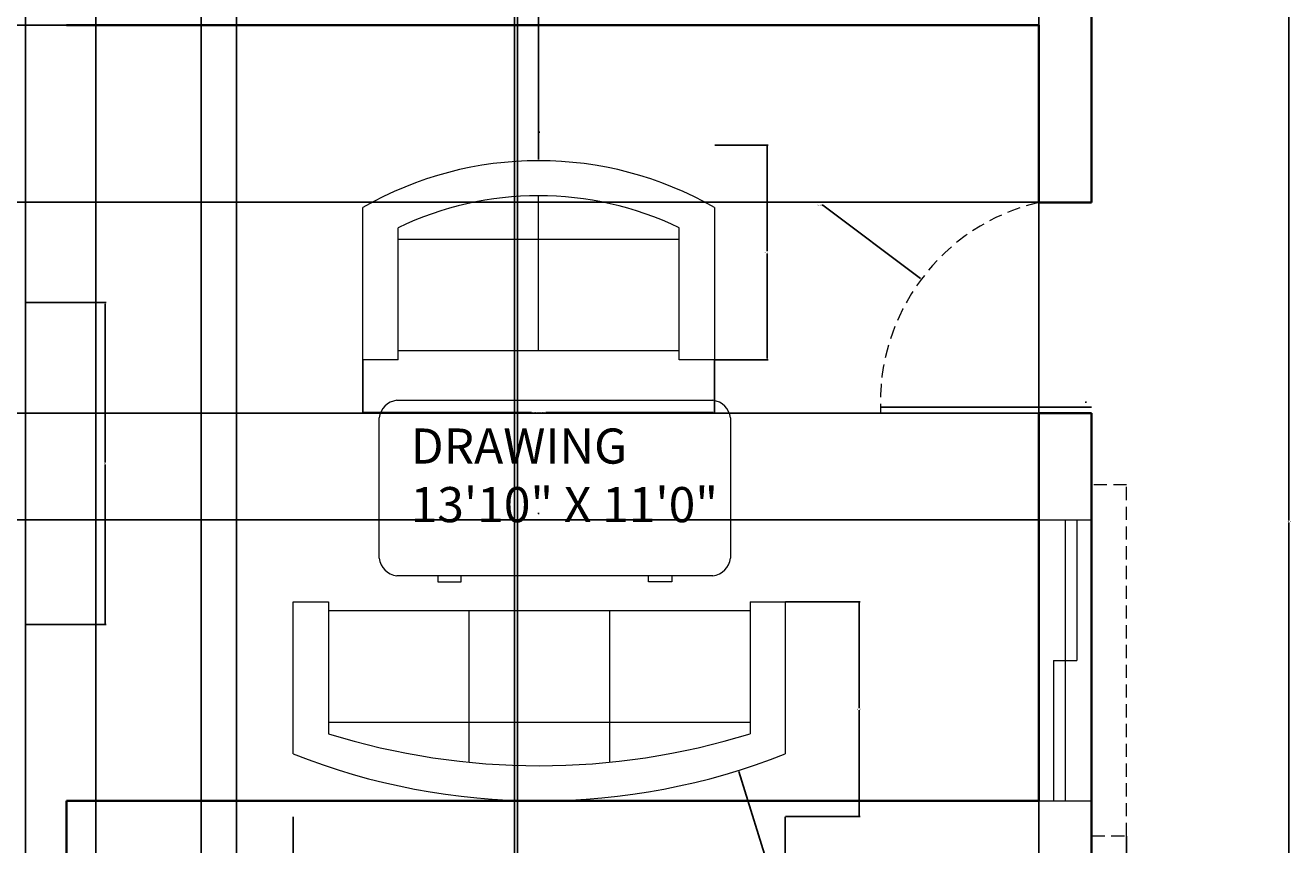
# Model space of a CAD drawing. Units: inches. Extents: x 6662 to 7211, y 5077 to 5683.
# Tile 6 of 9: x 6995 to 7211, y 5325 to 5465. Entities that reach past the tile are written whole.
import ezdxf

# ---------------------------------------------------------------- set-up
doc = ezdxf.new("R2010")
doc.units = ezdxf.units.IN
doc.header["$LTSCALE"] = 3
doc.header["$MEASUREMENT"] = 0
doc.linetypes.add('HIDDEN', pattern=[0.375, 0.25, -0.125])
for name, color, linetype, lineweight in [('A-ANNO-DIMS', 2, 'Continuous', 18), ('A-AREA-IDEN', 7, 'Continuous', 18), ('A-DOOR', 4, 'Continuous', 25), ('A-DOOR-HIDN', 4, 'HIDDEN', 13), ('A-FLOR-CASE-PATT', 241, 'Continuous', 13), ('A-FURN', 8, 'Continuous', 18), ('A-GLAZ', 4, 'Continuous', 18), ('A-GLAZ-OVHD', 4, 'HIDDEN', 13), ('A-WALL', 7, 'Continuous', 35)]:
    doc.layers.add(name, color=color, linetype=linetype, lineweight=lineweight)
doc.styles.get("Standard").update_dxf_attribs({"font": 'arial.ttf'})
doc.dimstyles.get("Standard").update_dxf_attribs({"dimtxt": 0.18, "dimasz": 0.18, "dimexe": 0.18, "dimexo": 0.0625, "dimgap": 0.09, "dimtad": 0, "dimtih": 1, "dimtoh": 1, "dimdec": 4, "dimzin": 0, "dimdsep": 46, "dimtxsty": 'Standard', "dimcen": 0.09, "dimadec": 0, "dimazin": 0, "dimtfac": 1, "dimtdec": 4, "dimtofl": 0, "dimtmove": 0, "dimatfit": 3, "dimfxl": 1, "dimtolj": 1, "dimtzin": 0, "dimarcsym": 0})

# ---------------------------------------------------------------- blocks, each defined once
blk = doc.blocks.new('Sofa - Roundback 7 ft.')
for p, q in [((-12.00002, -32.4421), (-12.00003, -6.5971)), ((11.99997, -32.4421), (11.99998, -6.5971)), ((-36.000027, -34), (-36.000027, -11.4696)), ((35.99998, -34), (35.99998, -11.4696)), ((-35.999844, -13.3819), (35.9998, -13.3819)), ((-36.000027, -32.4421), (35.99998, -32.4421))]:
    blk.add_line(p, q)
for points in [[(-36.000027, -34), (-42.000027, -34), (-42.000027, -8)], [(41.99998, -8), (41.99998, -34), (35.99998, -34)]]:
    blk.add_lwpolyline(points)
for centre, radius, start, end in [((0, -114.25), 114.25, 68.43141, 111.5686), ((-0.00001, -127.1968), 121.1968, 72.72033, 107.2797)]:
    blk.add_arc(centre, radius, start, end)
blk = doc.blocks.new('Desk - 30 x 60 in.')
for p, q in [((-26.999995, 0), (26.999995, 0)), ((-29.999995, -27), (-29.999995, -3)), ((29.999995, -3), (29.999995, -27)), ((26.999995, -30), (-26.999995, -30)), ((-20.000005, -30), (-20.000005, -31)), ((-16.000005, -31), (-16.000005, -30)), ((15.999995, -31), (15.999995, -30)), ((19.999995, -30), (19.999995, -31)), ((-20.000005, -31), (-16.000005, -31)), ((19.999995, -31), (15.999995, -31))]:
    blk.add_line(p, q)
for centre, start, end in [((-26.499995, -3.5), 98.1301, 171.8699), ((26.499995, -3.5), 8.130102, 81.8699), ((-26.499995, -26.5), 188.1301, 261.8699), ((26.499995, -26.5), 278.1301, 351.8699)]:
    blk.add_arc(centre, 3.535534, start, end)
blk = doc.blocks.new('Sofa - Roundback Loveseat 5 ft.')
for p, q in [((0, -32.44198), (0, -5.99998)), ((-24, -33.99998), (-24, -11.46958)), ((24.00004, -33.99998), (24.00004, -11.46958)), ((-23.9998, -13.38178), (23.99986, -13.38178)), ((-24, -32.44198), (24.00004, -32.44198))]:
    blk.add_line(p, q)
for points in [[(-24, -33.99998), (-30, -33.99998), (-30, -7.99998)], [(30.00004, -7.99998), (30.00004, -33.99998), (24.00004, -33.99998)]]:
    blk.add_lwpolyline(points)
for centre, radius, start, end in [((0, -60.24998), 60.24998, 60.13715, 119.8628), ((0, -61.38438), 55.38444, 64.32083, 115.6792)]:
    blk.add_arc(centre, radius, start, end)
blk = doc.blocks.new('WIN-SLIDER-48IN')
for p, q in [((0, 0), (0, 9)), ((48, 0), (48, 9)), ((0, 6.5), (24, 6.5)), ((24, 2.5), (24, 6.5)), ((0, 4.5), (48, 4.5)), ((24, 2.5), (48, 2.5))]:
    blk.add_line(p, q)
blk = doc.blocks.new('WIN-HOOD-48IN')
at = {"ltscale": 3}
for p, q in [((0, 0), (0, 6)), ((0, 6), (54, 6)), ((54, 6), (60, 6)), ((60, 6), (60, 0)), ((6, 0), (0, 0))]:
    blk.add_line(p, q, dxfattribs=at)
blk = doc.blocks.new('*D28')
at = {"layer": 'A-ANNO-DIMS', "color": 0, "lineweight": -2, "ltscale": 3, "transparency": 16777216}
for p, q in [((7040.57, 5329.37), (7040.57, 5316.65)), ((7124.57, 5329.37), (7124.57, 5316.65)), ((7040.75, 5316.83), (7081.66, 5316.83)), ((7124.39, 5316.83), (7083.47, 5316.83))]:
    blk.add_line(p, q, dxfattribs=at)
at = {"layer": 'A-ANNO-DIMS', "color": 0, "ltscale": 3, "transparency": 16777216}
for points in [[(7040.75, 5316.86), (7040.75, 5316.8), (7040.57, 5316.83)], [(7124.39, 5316.86), (7124.39, 5316.8), (7124.57, 5316.83)]]:
    blk.add_solid(points, dxfattribs=at)
at = {"layer": 'Defpoints', "color": 0, "ltscale": 3, "transparency": 16777216}
for p in [(7040.57, 5329.43), (7124.57, 5329.43), (7040.57, 5316.83)]:
    blk.add_point(p, dxfattribs=at)
at = {"layer": 'A-ANNO-DIMS', "color": 0, "ltscale": 3, "transparency": 16777216, "insert": (7082.57, 5316.83), "char_height": 0.18, "attachment_point": 5}
blk.add_mtext('\\A1;SOFA 84 TYP.', dxfattribs=at)
blk = doc.blocks.new('*D29')
at = {"layer": 'A-ANNO-DIMS', "color": 0, "lineweight": -2, "ltscale": 3, "transparency": 16777216}
for p, q in [((7124.63, 5366.1), (7137.35, 5366.1)), ((7137.17, 5365.92), (7137.17, 5347.95)), ((7137.17, 5329.61), (7137.17, 5347.58)), ((7124.63, 5329.43), (7137.35, 5329.43))]:
    blk.add_line(p, q, dxfattribs=at)
at = {"layer": 'A-ANNO-DIMS', "color": 0, "ltscale": 3, "transparency": 16777216}
for points in [[(7137.14, 5365.92), (7137.2, 5365.92), (7137.17, 5366.1)], [(7137.14, 5329.61), (7137.2, 5329.61), (7137.17, 5329.43)]]:
    blk.add_solid(points, dxfattribs=at)
at = {"layer": 'Defpoints', "color": 0, "ltscale": 3, "transparency": 16777216}
for p in [(7124.57, 5366.1), (7124.57, 5329.43), (7137.17, 5329.43)]:
    blk.add_point(p, dxfattribs=at)
at = {"layer": 'A-ANNO-DIMS', "color": 0, "ltscale": 3, "transparency": 16777216, "insert": (7137.17, 5347.76), "char_height": 0.18, "attachment_point": 5}
blk.add_mtext('\\A1;37 TYP.', dxfattribs=at)
blk = doc.blocks.new('*D32')
at = {"layer": 'A-ANNO-DIMS', "color": 0, "lineweight": -2, "ltscale": 3, "transparency": 16777216}
for p, q in [((7052.47, 5407.4), (7052.47, 5398.28)), ((7112.47, 5407.4), (7112.47, 5398.28)), ((7052.65, 5398.46), (7081.24, 5398.46)), ((7112.29, 5398.46), (7083.69, 5398.46))]:
    blk.add_line(p, q, dxfattribs=at)
at = {"layer": 'A-ANNO-DIMS', "color": 0, "ltscale": 3, "transparency": 16777216}
for points in [[(7052.65, 5398.49), (7052.65, 5398.43), (7052.47, 5398.46)], [(7112.29, 5398.49), (7112.29, 5398.43), (7112.47, 5398.46)]]:
    blk.add_solid(points, dxfattribs=at)
at = {"layer": 'Defpoints', "color": 0, "ltscale": 3, "transparency": 16777216}
for p in [(7052.47, 5407.46), (7112.47, 5407.46), (7112.47, 5398.46)]:
    blk.add_point(p, dxfattribs=at)
at = {"layer": 'A-ANNO-DIMS', "color": 0, "ltscale": 3, "transparency": 16777216, "insert": (7082.47, 5398.46), "char_height": 0.18, "attachment_point": 5}
blk.add_mtext('\\A1;LOVESEAT 60 TYP.', dxfattribs=at)
blk = doc.blocks.new('*D33')
at = {"layer": 'A-ANNO-DIMS', "color": 0, "lineweight": -2, "ltscale": 3, "transparency": 16777216}
for p, q in [((7112.53, 5444.13), (7121.65, 5444.13)), ((7121.47, 5443.95), (7121.47, 5425.98)), ((7121.47, 5407.64), (7121.47, 5425.61)), ((7112.53, 5407.46), (7121.65, 5407.46))]:
    blk.add_line(p, q, dxfattribs=at)
at = {"layer": 'A-ANNO-DIMS', "color": 0, "ltscale": 3, "transparency": 16777216}
for points in [[(7121.44, 5443.95), (7121.5, 5443.95), (7121.47, 5444.13)], [(7121.44, 5407.64), (7121.5, 5407.64), (7121.47, 5407.46)]]:
    blk.add_solid(points, dxfattribs=at)
at = {"layer": 'Defpoints', "color": 0, "ltscale": 3, "transparency": 16777216}
for p in [(7112.47, 5444.13), (7121.47, 5444.13), (7112.47, 5407.46)]:
    blk.add_point(p, dxfattribs=at)
at = {"layer": 'A-ANNO-DIMS', "color": 0, "ltscale": 3, "transparency": 16777216, "insert": (7121.47, 5425.8), "char_height": 0.18, "attachment_point": 5}
blk.add_mtext('\\A1;37 TYP.', dxfattribs=at)
blk = doc.blocks.new('*D39')
at = {"layer": 'A-ANNO-DIMS', "color": 0, "lineweight": -2, "ltscale": 3, "transparency": 16777216}
for p, q in [((6994.86, 5417.21), (7008.62, 5417.21)), ((7008.44, 5417.03), (7008.44, 5389.9)), ((7008.44, 5362.39), (7008.44, 5389.53)), ((6994.86, 5362.21), (7008.62, 5362.21))]:
    blk.add_line(p, q, dxfattribs=at)
at = {"layer": 'A-ANNO-DIMS', "color": 0, "ltscale": 3, "transparency": 16777216}
for points in [[(7008.41, 5417.03), (7008.47, 5417.03), (7008.44, 5417.21)], [(7008.41, 5362.39), (7008.47, 5362.39), (7008.44, 5362.21)]]:
    blk.add_solid(points, dxfattribs=at)
at = {"layer": 'Defpoints', "color": 0, "ltscale": 3, "transparency": 16777216}
for p in [(6994.79, 5417.21), (7008.44, 5417.21), (6994.79, 5362.21)]:
    blk.add_point(p, dxfattribs=at)
at = {"layer": 'A-ANNO-DIMS', "color": 0, "ltscale": 3, "transparency": 16777216, "insert": (7008.44, 5389.71), "char_height": 0.18, "attachment_point": 5}
blk.add_mtext('\\A1;55', dxfattribs=at)
blk = doc.blocks.new('*D40')
at = {"layer": 'A-ANNO-DIMS', "color": 0, "lineweight": -2, "ltscale": 3, "transparency": 16777216}
for p, q in [((7182.86, 5326.04), (7182.86, 5076.72)), ((6689.86, 5323.04), (6689.86, 5076.72)), ((6690.04, 5076.9), (6936.07, 5076.9)), ((7182.68, 5076.9), (6936.65, 5076.9))]:
    blk.add_line(p, q, dxfattribs=at)
at = {"layer": 'A-ANNO-DIMS', "color": 0, "ltscale": 3, "transparency": 16777216}
for points in [[(6690.04, 5076.93), (6690.04, 5076.87), (6689.86, 5076.9)], [(7182.68, 5076.93), (7182.68, 5076.87), (7182.86, 5076.9)]]:
    blk.add_solid(points, dxfattribs=at)
at = {"layer": 'Defpoints', "color": 0, "ltscale": 3, "transparency": 16777216}
for p in [(7182.86, 5326.1), (6689.86, 5323.1), (7182.86, 5076.9)]:
    blk.add_point(p, dxfattribs=at)
at = {"layer": 'A-ANNO-DIMS', "color": 0, "ltscale": 3, "transparency": 16777216, "insert": (6936.36, 5076.9), "char_height": 0.18, "attachment_point": 5}
blk.add_mtext('\\A1;493', dxfattribs=at)
blk = doc.blocks.new('*D41')
at = {"layer": 'A-ANNO-DIMS', "color": 0, "lineweight": -2, "ltscale": 3, "transparency": 16777216}
for p, q in [((7035.92, 5655.02), (7210.74, 5655.02)), ((7210.56, 5654.84), (7210.56, 5379.99)), ((7210.56, 5104.78), (7210.56, 5379.63)), ((7010.92, 5104.6), (7210.74, 5104.6))]:
    blk.add_line(p, q, dxfattribs=at)
at = {"layer": 'A-ANNO-DIMS', "color": 0, "ltscale": 3, "transparency": 16777216}
for points in [[(7210.53, 5654.84), (7210.59, 5654.84), (7210.56, 5655.02)], [(7210.53, 5104.78), (7210.59, 5104.78), (7210.56, 5104.6)]]:
    blk.add_solid(points, dxfattribs=at)
at = {"layer": 'Defpoints', "color": 0, "ltscale": 3, "transparency": 16777216}
for p in [(7035.86, 5655.02), (7210.56, 5655.02), (7010.86, 5104.6)]:
    blk.add_point(p, dxfattribs=at)
at = {"layer": 'A-ANNO-DIMS', "color": 0, "ltscale": 3, "transparency": 16777216, "insert": (7210.56, 5379.81), "char_height": 0.18, "attachment_point": 5}
blk.add_mtext('\\A1;550.4', dxfattribs=at)
blk = doc.blocks.new('*D61')
at = {"layer": 'A-ANNO-DIMS', "color": 0, "lineweight": -2, "ltscale": 3, "transparency": 16777216}
for p, q in [((7167.8, 5434.35), (6661.98, 5434.35)), ((6662.16, 5434.17), (6662.16, 5416.53)), ((6662.16, 5398.53), (6662.16, 5416.17)), ((7167.8, 5398.35), (6661.98, 5398.35))]:
    blk.add_line(p, q, dxfattribs=at)
at = {"layer": 'A-ANNO-DIMS', "color": 0, "ltscale": 3, "transparency": 16777216}
for points in [[(6662.13, 5434.17), (6662.19, 5434.17), (6662.16, 5434.35)], [(6662.13, 5398.53), (6662.19, 5398.53), (6662.16, 5398.35)]]:
    blk.add_solid(points, dxfattribs=at)
at = {"layer": 'Defpoints', "color": 0, "ltscale": 3, "transparency": 16777216}
for p in [(6662.16, 5434.35), (7167.86, 5434.35), (7167.86, 5398.35)]:
    blk.add_point(p, dxfattribs=at)
at = {"layer": 'A-ANNO-DIMS', "color": 0, "ltscale": 3, "transparency": 16777216, "insert": (6662.16, 5416.35), "char_height": 0.18, "attachment_point": 5}
blk.add_mtext('\\A1;36', dxfattribs=at)
blk = doc.blocks.new('*D67')
at = {"layer": 'A-ANNO-DIMS', "color": 0, "lineweight": -2, "ltscale": 3, "transparency": 16777216}
for p, q in [((6994.86, 5514.54), (6994.86, 5076.72)), ((7024.86, 5514.54), (7024.86, 5076.72)), ((6995.04, 5076.9), (7009.64, 5076.9)), ((7024.68, 5076.9), (7010.08, 5076.9))]:
    blk.add_line(p, q, dxfattribs=at)
at = {"layer": 'A-ANNO-DIMS', "color": 0, "ltscale": 3, "transparency": 16777216}
for points in [[(6995.04, 5076.93), (6995.04, 5076.87), (6994.86, 5076.9)], [(7024.68, 5076.93), (7024.68, 5076.87), (7024.86, 5076.9)]]:
    blk.add_solid(points, dxfattribs=at)
at = {"layer": 'Defpoints', "color": 0, "ltscale": 3, "transparency": 16777216}
for p in [(6994.86, 5514.6), (7024.86, 5514.6), (7024.86, 5076.9)]:
    blk.add_point(p, dxfattribs=at)
at = {"layer": 'A-ANNO-DIMS', "color": 0, "ltscale": 3, "transparency": 16777216, "insert": (7009.86, 5076.9), "char_height": 0.18, "attachment_point": 5}
blk.add_mtext('\\A1;30', dxfattribs=at)
blk = doc.blocks.new('*D74')
at = {"layer": 'A-ANNO-DIMS', "color": 0, "lineweight": -2, "ltscale": 3, "transparency": 16777216}
for p, q in [((7006.86, 5179.16), (7006.86, 5682.9)), ((7007.04, 5682.72), (7018.64, 5682.72)), ((7030.68, 5682.72), (7019.08, 5682.72)), ((7030.86, 5179.16), (7030.86, 5682.9))]:
    blk.add_line(p, q, dxfattribs=at)
at = {"layer": 'A-ANNO-DIMS', "color": 0, "ltscale": 3, "transparency": 16777216}
for points in [[(7007.04, 5682.75), (7007.04, 5682.69), (7006.86, 5682.72)], [(7030.68, 5682.75), (7030.68, 5682.69), (7030.86, 5682.72)]]:
    blk.add_solid(points, dxfattribs=at)
at = {"layer": 'Defpoints', "color": 0, "ltscale": 3, "transparency": 16777216}
for p in [(7030.86, 5682.72), (7006.86, 5179.1), (7030.86, 5179.1)]:
    blk.add_point(p, dxfattribs=at)
at = {"layer": 'A-ANNO-DIMS', "color": 0, "ltscale": 3, "transparency": 16777216, "insert": (7018.86, 5682.72), "char_height": 0.18, "attachment_point": 5}
blk.add_mtext('\\A1;24', dxfattribs=at)
blk = doc.blocks.new('*D75')
at = {"layer": 'A-ANNO-DIMS', "color": 0, "lineweight": -2, "ltscale": 3, "transparency": 16777216}
for p, q in [((7030.86, 5179.16), (7030.86, 5682.9)), ((7031.04, 5682.72), (7054.64, 5682.72)), ((7078.68, 5682.72), (7055.08, 5682.72)), ((7078.86, 5179.16), (7078.86, 5682.9))]:
    blk.add_line(p, q, dxfattribs=at)
at = {"layer": 'A-ANNO-DIMS', "color": 0, "ltscale": 3, "transparency": 16777216}
for points in [[(7031.04, 5682.75), (7031.04, 5682.69), (7030.86, 5682.72)], [(7078.68, 5682.75), (7078.68, 5682.69), (7078.86, 5682.72)]]:
    blk.add_solid(points, dxfattribs=at)
at = {"layer": 'Defpoints', "color": 0, "ltscale": 3, "transparency": 16777216}
for p in [(7078.86, 5682.72), (7030.86, 5179.1), (7078.86, 5179.1)]:
    blk.add_point(p, dxfattribs=at)
at = {"layer": 'A-ANNO-DIMS', "color": 0, "ltscale": 3, "transparency": 16777216, "insert": (7054.86, 5682.72), "char_height": 0.18, "attachment_point": 5}
blk.add_mtext('\\A1;48', dxfattribs=at)
blk = doc.blocks.new('*D76')
at = {"layer": 'A-ANNO-DIMS', "color": 0, "lineweight": -2, "ltscale": 3, "transparency": 16777216}
for p, q in [((7167.8, 5464.6), (6661.98, 5464.6)), ((6662.16, 5464.42), (6662.16, 5449.65)), ((6662.16, 5434.53), (6662.16, 5449.29)), ((7167.8, 5434.35), (6661.98, 5434.35))]:
    blk.add_line(p, q, dxfattribs=at)
at = {"layer": 'A-ANNO-DIMS', "color": 0, "ltscale": 3, "transparency": 16777216}
for points in [[(6662.13, 5464.42), (6662.19, 5464.42), (6662.16, 5464.6)], [(6662.13, 5434.53), (6662.19, 5434.53), (6662.16, 5434.35)]]:
    blk.add_solid(points, dxfattribs=at)
at = {"layer": 'Defpoints', "color": 0, "ltscale": 3, "transparency": 16777216}
for p in [(7167.86, 5464.6), (6662.16, 5434.35), (7167.86, 5434.35)]:
    blk.add_point(p, dxfattribs=at)
at = {"layer": 'A-ANNO-DIMS', "color": 0, "ltscale": 3, "transparency": 16777216, "insert": (6662.16, 5449.47), "char_height": 0.18, "attachment_point": 5}
blk.add_mtext('\\A1;30.25', dxfattribs=at)
blk = doc.blocks.new('*D77')
at = {"layer": 'A-ANNO-DIMS', "color": 0, "lineweight": -2, "ltscale": 3, "transparency": 16777216}
for p, q in [((7167.8, 5398.35), (6661.98, 5398.35)), ((6662.16, 5398.17), (6662.16, 5389.4)), ((6662.16, 5380.28), (6662.16, 5389.04)), ((7167.8, 5380.1), (6661.98, 5380.1))]:
    blk.add_line(p, q, dxfattribs=at)
at = {"layer": 'A-ANNO-DIMS', "color": 0, "ltscale": 3, "transparency": 16777216}
for points in [[(6662.13, 5398.17), (6662.19, 5398.17), (6662.16, 5398.35)], [(6662.13, 5380.28), (6662.19, 5380.28), (6662.16, 5380.1)]]:
    blk.add_solid(points, dxfattribs=at)
at = {"layer": 'Defpoints', "color": 0, "ltscale": 3, "transparency": 16777216}
for p in [(7167.86, 5398.35), (6662.16, 5380.1), (7167.86, 5380.1)]:
    blk.add_point(p, dxfattribs=at)
at = {"layer": 'A-ANNO-DIMS', "color": 0, "ltscale": 3, "transparency": 16777216, "insert": (6662.16, 5389.22), "char_height": 0.18, "attachment_point": 5}
blk.add_mtext('\\A1;18.25', dxfattribs=at)
blk = doc.blocks.new('*D81')
at = {"layer": 'A-ANNO-DIMS', "color": 0, "lineweight": -2, "ltscale": 3, "transparency": 16777216}
for p, q in [((7078.36, 5473.54), (7078.36, 5076.72)), ((7167.86, 5473.54), (7167.86, 5076.72)), ((7078.54, 5076.9), (7122.78, 5076.9)), ((7167.68, 5076.9), (7123.43, 5076.9))]:
    blk.add_line(p, q, dxfattribs=at)
at = {"layer": 'A-ANNO-DIMS', "color": 0, "ltscale": 3, "transparency": 16777216}
for points in [[(7078.54, 5076.93), (7078.54, 5076.87), (7078.36, 5076.9)], [(7167.68, 5076.93), (7167.68, 5076.87), (7167.86, 5076.9)]]:
    blk.add_solid(points, dxfattribs=at)
at = {"layer": 'Defpoints', "color": 0, "ltscale": 3, "transparency": 16777216}
for p in [(7078.36, 5473.6), (7167.86, 5473.6), (7167.86, 5076.9)]:
    blk.add_point(p, dxfattribs=at)
at = {"layer": 'A-ANNO-DIMS', "color": 0, "ltscale": 3, "transparency": 16777216, "insert": (7123.11, 5076.9), "char_height": 0.18, "attachment_point": 5}
blk.add_mtext('\\A1;89.5', dxfattribs=at)
blk = doc.blocks.new('*D89')
at = {"layer": 'A-ANNO-DIMS', "color": 0, "lineweight": -2, "ltscale": 3, "transparency": 16777216}
for p, q in [((7130.8, 5433.88), (7130.98, 5433.88)), ((7130.98, 5433.88), (7147.68, 5421.35)), ((7175.82, 5400.19), (7176, 5400.19)), ((7175.91, 5400.1), (7175.91, 5400.28))]:
    blk.add_line(p, q, dxfattribs=at)
at = {"layer": 'A-ANNO-DIMS', "color": 0, "ltscale": 3, "transparency": 16777216}
blk.add_solid([(7147.7, 5421.38), (7147.67, 5421.33), (7147.83, 5421.25)], dxfattribs=at)
at = {"layer": 'Defpoints', "color": 0, "ltscale": 3, "transparency": 16777216}
for p in [(7147.83, 5421.25), (7175.91, 5400.19)]:
    blk.add_point(p, dxfattribs=at)
at = {"layer": 'A-ANNO-DIMS', "color": 0, "ltscale": 3, "transparency": 16777216, "insert": (7130.25, 5433.88), "char_height": 0.18, "attachment_point": 5}
blk.add_mtext('\\A1;R35.095', dxfattribs=at)
blk = doc.blocks.new('*D101')
at = {"layer": 'A-ANNO-DIMS', "color": 0, "lineweight": -2, "ltscale": 3, "transparency": 16777216}
for p, q in [((7082.48, 5446.35), (7082.66, 5446.35)), ((7082.57, 5446.26), (7082.57, 5446.44)), ((7136.97, 5271.83), (7116.62, 5337.1)), ((7137.15, 5271.83), (7136.97, 5271.83))]:
    blk.add_line(p, q, dxfattribs=at)
at = {"layer": 'A-ANNO-DIMS', "color": 0, "ltscale": 3, "transparency": 16777216}
blk.add_solid([(7116.65, 5337.11), (7116.6, 5337.09), (7116.57, 5337.27)], dxfattribs=at)
at = {"layer": 'Defpoints', "color": 0, "ltscale": 3, "transparency": 16777216}
for p in [(7082.57, 5446.35), (7116.57, 5337.27)]:
    blk.add_point(p, dxfattribs=at)
at = {"layer": 'A-ANNO-DIMS', "color": 0, "ltscale": 3, "transparency": 16777216, "insert": (7137.9, 5271.83), "char_height": 0.18, "attachment_point": 5}
blk.add_mtext('\\A1;2X R114.25', dxfattribs=at)
blk = doc.blocks.new('*D103')
at = {"layer": 'A-ANNO-DIMS', "color": 0, "lineweight": -2, "ltscale": 3, "transparency": 16777216}
for p, q in [((7082.65, 5477.61), (7082.47, 5477.61)), ((7082.47, 5477.61), (7082.47, 5441.64)), ((7082.38, 5381.21), (7082.56, 5381.21)), ((7082.47, 5381.12), (7082.47, 5381.3))]:
    blk.add_line(p, q, dxfattribs=at)
at = {"layer": 'A-ANNO-DIMS', "color": 0, "ltscale": 3, "transparency": 16777216}
blk.add_solid([(7082.44, 5441.64), (7082.5, 5441.64), (7082.47, 5441.46)], dxfattribs=at)
at = {"layer": 'Defpoints', "color": 0, "ltscale": 3, "transparency": 16777216}
for p in [(7082.47, 5441.46), (7082.47, 5381.21)]:
    blk.add_point(p, dxfattribs=at)
at = {"layer": 'A-ANNO-DIMS', "color": 0, "ltscale": 3, "transparency": 16777216, "insert": (7083.32, 5477.61), "char_height": 0.18, "attachment_point": 5}
blk.add_mtext('\\A1;2X R60.25', dxfattribs=at)

msp = doc.modelspace()

# ---------------------------------------------------------------- hatches: boundary and pattern name
at = {"layer": 'A-FLOR-CASE-PATT'}
h = msp.add_hatch(dxfattribs=at)
h.set_pattern_fill('ANSI31', color=256)
h.paths.add_polyline_path([(6869.8579, 5283.7981), (6845.8579, 5283.7981), (6845.8579, 5229.4653), (6847.018, 5229.7817, -0.54116316), (6849.0925, 5228.1371), (6849.7129, 5228.234, -0.50821327), (6851.018, 5227.2817), (6851.018, 5226.7817), (6855.018, 5227.2817), (6855.018, 5225.7817), (6851.018, 5225.2817), (6851.018, 5217.7817), (6851.018, 5210.2817), (6855.018, 5209.7817), (6855.018, 5208.2817), (6851.018, 5208.7817), (6851.018, 5208.2817, -0.41421356), (6850.018, 5207.2817), (6849.0925, 5207.4263, -0.50580924), (6847.1872, 5205.7355), (6845.8579, 5206.0981), (6845.8579, 5179.0979), (6869.8579, 5179.0979)])
h.paths.add_polyline_path([(7167.8579, 5497.5979), (7143.8579, 5497.5979), (7078.3579, 5497.5979), (7078.3579, 5473.5979), (7163.8579, 5473.5979), (7167.8579, 5473.5979)])
h.paths.add_polyline_path([(6825.9016, 5497.5979), (6725.8579, 5497.5979), (6725.8579, 5473.5979), (6825.9016, 5473.5979)])
h.paths.add_polyline_path([(6796.6359, 5485.2095), (6797.1359, 5489.2095), (6806.1359, 5489.2095), (6815.1359, 5489.2095), (6815.6359, 5485.2095), (6814.1359, 5485.2095), (6813.6359, 5489.2095), (6806.1359, 5489.2095), (6798.6359, 5489.2095), (6798.1359, 5485.2095)], flags=16)

# ---------------------------------------------------------------- linework, layer by layer
at = {"layer": 'A-DOOR'}
for p, q in [((7176.8579, 5399.3479), (7140.8579, 5399.3479)), ((7176.8579, 5398.3479), (7140.8579, 5398.3479))]:
    msp.add_line(p, q, dxfattribs=at)
at = {"layer": 'A-DOOR-HIDN', "ltscale": 3}
msp.add_arc((7175.9051, 5400.1875), 35.0955, 103.255569, 183.004636, dxfattribs=at)
at = {"layer": 'A-WALL'}
for p, q in [((7176.8579, 5434.3479), (7176.8579, 5626.5979)), ((7167.8579, 5464.5979), (7001.8579, 5464.5979)), ((7167.8579, 5434.3479), (7167.8579, 5464.5979)), ((7167.8579, 5434.3479), (7167.8579, 5464.5979)), ((7167.8579, 5434.3479), (7176.8579, 5434.3479)), ((7167.8579, 5332.0979), (7167.8579, 5398.3479)), ((7167.8579, 5332.0979), (7167.8579, 5398.3479)), ((7167.8579, 5398.3479), (7176.8579, 5398.3479)), ((7176.8579, 5170.0979), (7176.8579, 5398.3479)), ((7106.8579, 5332.0979), (7001.8579, 5332.0979)), ((7001.8579, 5323.0979), (7001.8579, 5332.0979)), ((7001.8579, 5323.0979), (7001.8579, 5332.0979)), ((7167.8579, 5332.0979), (7010.8579, 5332.0979))]:
    msp.add_line(p, q, dxfattribs=at)

# ---------------------------------------------------------------- block references
at = {"layer": 'A-FURN'}
for name, p in [('Sofa - Roundback Loveseat 5 ft.', (7082.466, 5441.4635)), ('Desk - 30 x 60 in.', (7085.2297, 5400.5342))]:
    msp.add_blockref(name, p, dxfattribs=at)
at = {"layer": 'A-FURN', "rotation": 180}
msp.add_blockref('Sofa - Roundback 7 ft.', (7082.5693, 5332.0979), dxfattribs=at)
at = {"layer": 'A-GLAZ', "rotation": 269.9999999999941}
msp.add_blockref('WIN-SLIDER-48IN', (7167.8579, 5380.0978), dxfattribs=at)
at = {"layer": 'A-GLAZ-OVHD', "extrusion": (0, 0, -1), "zscale": -1, "rotation": 89.99999999999515}
msp.add_blockref('WIN-HOOD-48IN', (-7176.8579, 5326.0981), dxfattribs=at)

# ---------------------------------------------------------------- texts
at = {"layer": 'A-AREA-IDEN', "ltscale": 3, "insert": (7060.6209, 5395.7092), "char_height": 6, "attachment_point": 1}
msp.add_mtext_dynamic_manual_height_columns('DRAWING\\P13\'10" X 11\'0"', width=381.547883, gutter_width=1, heights=[0], dxfattribs=at)

# ---------------------------------------------------------------- dimensions: what is measured, and where the dimension line sits
at = {"layer": 'A-ANNO-DIMS', "ltscale": 3}
for base, p1, p2, override, picture, middle in [((7030.8579, 5682.7209), (7006.8579, 5179.0979), (7030.8579, 5179.0979), {"dimdec": 0, "dimlfac": 1, "dimrnd": 0, "dimzin": 0, "dimdsep": 46, "dimlunit": 2}, '*D74', (7018.8579, 5682.7209)), ((7078.8579, 5682.7209), (7030.8579, 5179.0979), (7078.8579, 5179.0979), {"dimdec": 0, "dimlfac": 1, "dimrnd": 0, "dimzin": 0, "dimdsep": 46, "dimlunit": 2}, '*D75', (7054.8579, 5682.7209)), ((7024.8579, 5076.8979), (6994.8579, 5514.5979), (7024.8579, 5514.5979), {"dimdec": 0, "dimlfac": 1, "dimrnd": 0, "dimzin": 0, "dimdsep": 46, "dimlunit": 2}, '*D67', (7009.8579, 5076.8979)), ((7167.8579, 5076.8979), (7078.3579, 5473.5979), (7167.8579, 5473.5979), {"dimdec": 1, "dimlfac": 1, "dimrnd": 0, "dimzin": 0, "dimdsep": 46, "dimlunit": 2}, '*D81', (7123.1079, 5076.8979)), ((7182.8579, 5076.8979), (6689.8579, 5323.0979), (7182.8579, 5326.0979), {"dimdec": 0, "dimlfac": 1, "dimrnd": 0, "dimzin": 0, "dimdsep": 46, "dimlunit": 2}, '*D40', (6936.3579, 5076.8979))]:
    dim = msp.add_linear_dim(base=base, p1=p1, p2=p2, dimstyle='Standard', override=override, dxfattribs=at)
    dim.commit()
    dim.dimension.update_dxf_attribs({"geometry": picture, "text_midpoint": middle})
for base, p1, p2, override, picture, middle in [((7210.5579, 5655.0209), (7010.8579, 5104.5979), (7035.8579, 5655.0209), {"dimdec": 1, "dimlfac": 1, "dimrnd": 0, "dimzin": 0, "dimdsep": 46, "dimlunit": 2}, '*D41', (7210.5579, 5379.8094)), ((6662.1579, 5434.3479), (7167.8579, 5464.5979), (7167.8579, 5434.3479), {"dimdec": 2, "dimlfac": 1, "dimrnd": 0, "dimzin": 0, "dimdsep": 46, "dimlunit": 2}, '*D76', (6662.1579, 5449.4729)), ((6662.1579, 5434.3479), (7167.8579, 5398.3479), (7167.8579, 5434.3479), {"dimdec": 0, "dimlfac": 1, "dimrnd": 0, "dimzin": 0, "dimdsep": 46, "dimlunit": 2}, '*D61', (6662.1579, 5416.3479)), ((7008.4433, 5417.2146), (6994.7933, 5362.2146), (6994.7933, 5417.2146), {"dimdec": 0, "dimlfac": 1, "dimrnd": 0, "dimzin": 0, "dimdsep": 46, "dimlunit": 2}, '*D39', (7008.4433, 5389.7146)), ((6662.1579, 5380.0979), (7167.8579, 5398.3479), (7167.8579, 5380.0979), {"dimdec": 2, "dimlfac": 1, "dimrnd": 0, "dimzin": 0, "dimdsep": 46, "dimlunit": 2}, '*D77', (6662.1579, 5389.2229))]:
    dim = msp.add_linear_dim(base=base, p1=p1, p2=p2, angle=90, dimstyle='Standard', override=override, dxfattribs=at)
    dim.commit()
    dim.dimension.update_dxf_attribs({"geometry": picture, "text_midpoint": middle})
for center, mpoint, picture, middle in [((7082.466, 5381.2135), (7082.466, 5441.4635), '*D103', (7083.3214, 5477.6135)), ((7082.5693, 5446.3479), (7116.5707, 5337.2747), '*D101', (7137.8968, 5271.8308))]:
    dim = msp.add_radius_dim(center=center, mpoint=mpoint, text='2X <>', dimstyle='Standard', override={"dimdec": 2, "dimlfac": 1, "dimrnd": 0, "dimzin": 0, "dimdsep": 46, "dimlunit": 2}, dxfattribs=at)
    dim.commit()
    dim.dimension.update_dxf_attribs({"geometry": picture, "text_midpoint": middle, "dimtype": 164})
for base, p1, p2, angle, text, picture, middle in [((7121.466, 5444.1302), (7112.466, 5407.4635), (7112.466, 5444.1302), 90, '<> TYP.', '*D33', (7121.466, 5425.7968)), ((7137.1694, 5329.4313), (7124.5694, 5366.0979), (7124.5694, 5329.4313), 270, '<> TYP.', '*D29', (7137.1694, 5347.7646)), ((7040.5693, 5316.8313), (7124.5694, 5329.4313), (7040.5693, 5329.4313), 180, 'SOFA <> TYP.', '*D28', (7082.5693, 5316.8313))]:
    dim = msp.add_linear_dim(base=base, p1=p1, p2=p2, angle=angle, text=text, dimstyle='Standard', override={"dimdec": 0, "dimlfac": 1, "dimrnd": 0, "dimzin": 0, "dimdsep": 46, "dimlunit": 2}, dxfattribs=at)
    dim.commit()
    dim.dimension.update_dxf_attribs({"geometry": picture, "text_midpoint": middle})
dim = msp.add_radius_dim(center=(7175.90508, 5400.18753), mpoint=(7147.82891, 5421.24507), dimstyle='Standard', override={"dimdec": 3, "dimlfac": 1, "dimrnd": 0, "dimzin": 0, "dimdsep": 46, "dimlunit": 2}, dxfattribs=at)
dim.commit()
dim.dimension.update_dxf_attribs({"geometry": '*D89', "text_midpoint": (7130.25277, 5433.87959), "dimtype": 164})
dim = msp.add_linear_dim(base=(7112.466, 5398.4635), p1=(7052.466, 5407.4635), p2=(7112.466, 5407.4635), text='LOVESEAT <> TYP.', dimstyle='Standard', override={"dimdec": 0, "dimlfac": 1, "dimrnd": 0, "dimzin": 0, "dimdsep": 46, "dimlunit": 2}, dxfattribs=at)
dim.commit()
dim.dimension.update_dxf_attribs({"geometry": '*D32', "text_midpoint": (7082.466, 5398.4635)})

doc.saveas('drawing.dxf')
